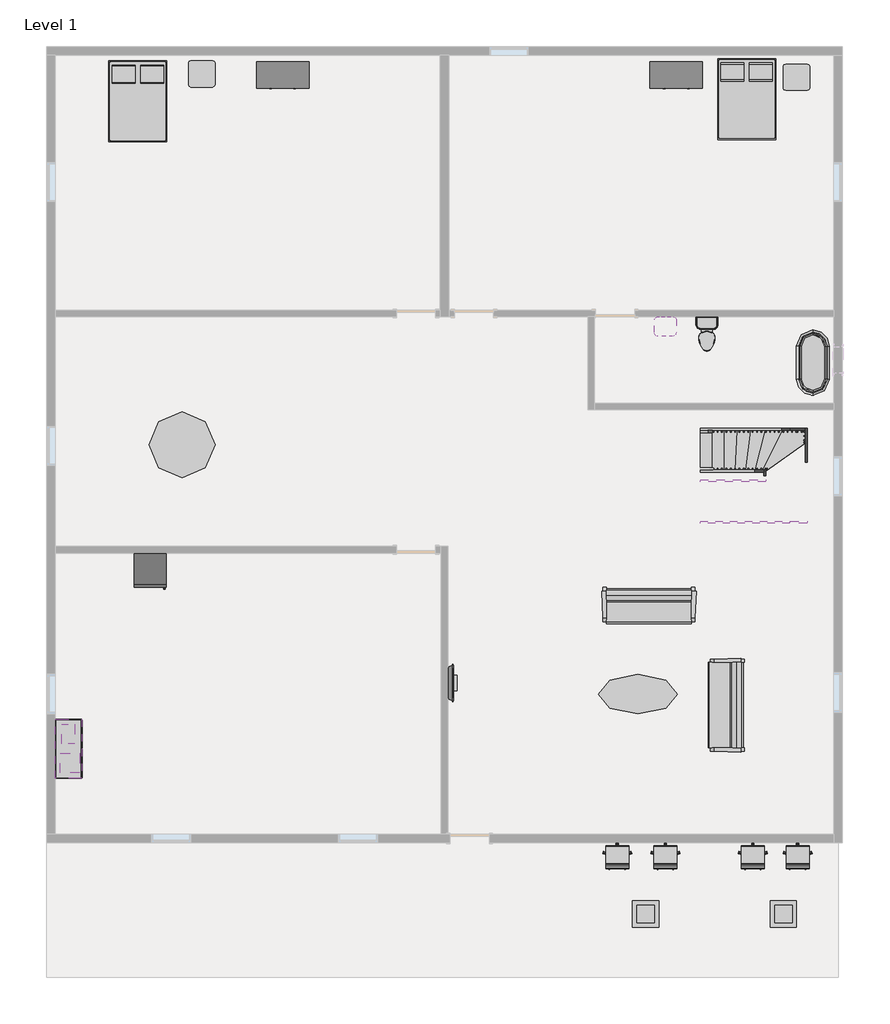
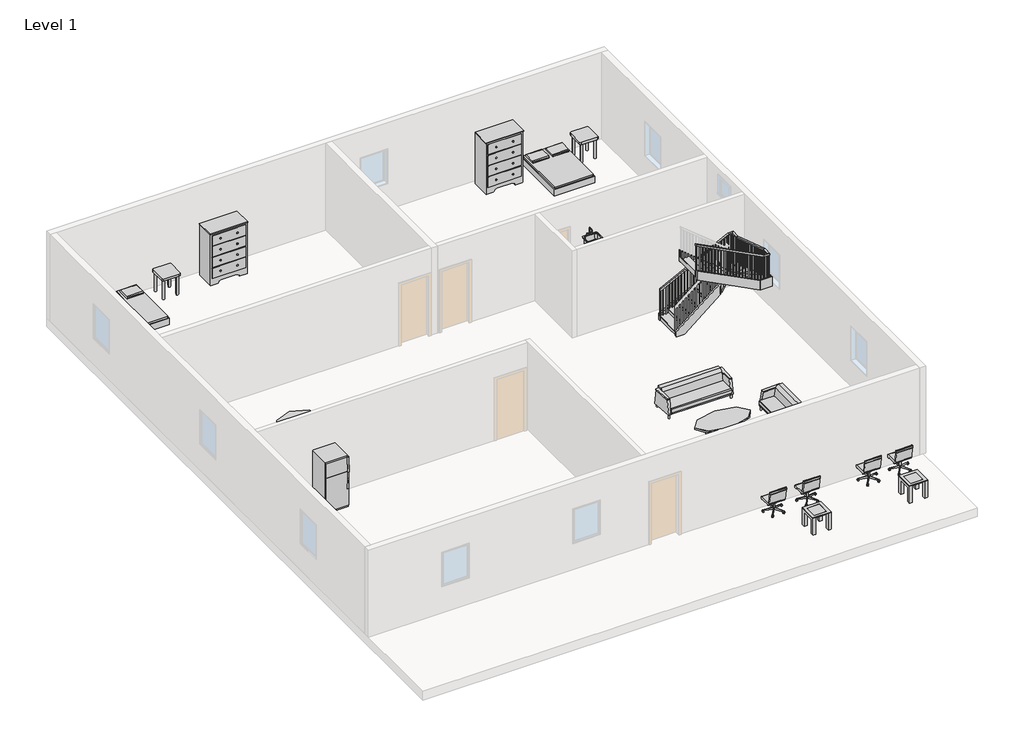
# One storey, part 2 of 2: 18 furniture elements, 8 members, 4 flow terminals, 3 proxies, 1 railing, 1 stair flight.
"""IFC4 building model written with IfcOpenShell, lengths in millimetres."""

from ifc_helpers import new_model, si_unit, frame, origin, place, context, project, spatial, polyline, outline, extrude, faceted_brep, transform, mapped, element, save
from components import proxy_fe84b772, proxy_844211aa, proxy_a13a33b2, flow_terminal_871c2e40, flow_terminal_62a433f7, toilet_domestic_3d_toilet_domestic_3d_f7549cf7, toilet_domestic_3d_toilet_domestic_3d_183bbd19, flow_terminal_b374fae2, furniture_c8abb964, chair_task_chair_task_b7f3823b, furniture_95afb093, furniture_9fa109b2, furniture_aff9b2fb, furniture_56245f3a, furniture_b5c51a22, furniture_bbcc68ce, furniture_027a2ad9, furniture_bcf351fa, stair_flight_58f01264

model = new_model("IFC4")

# Units and contexts
model_context = context("Model", 3, world=origin())
ifc_project = project(units=[si_unit("LENGTHUNIT", "METRE", prefix="MILLI")], contexts=[model_context])

# Site, building, storey
site = spatial("IfcSite", under=ifc_project)
building = spatial("IfcBuilding", under=site)
storey = spatial("IfcBuildingStorey", under=building, Name="Level 1", Elevation=0.0)

# Proxies
placement = place(None, origin())
proxy_shape = proxy_fe84b772(model_context)
element("IfcBuildingElementProxy", 1, Name="Cook Top-2 Unit : 12\" x 18\"", ObjectType="Cook Top-2 Unit : 12\" x 18\"", at=placement, inside=storey, context=model_context, shape_type="MappedRepresentation", body=[
    mapped(proxy_shape, transform((-16052.9808972, -1489.9035107, 914.4), x_axis=(-1.0000000000000002, 0.0, 0.0), y_axis=(0.0, -1.0000000000000002, 0.0), z_axis=(0.0, 0.0, 1.0))),
])
proxy_2_shape = proxy_844211aa(model_context)
element("IfcBuildingElementProxy", 2, Name="Kitchenette - Small : 54\"", ObjectType="Kitchenette - Small : 54\"", at=placement, inside=storey, context=model_context, shape_type="MappedRepresentation", body=[
    mapped(proxy_2_shape, transform((-16433.9808972, -1881.7660112, 914.4), x_axis=(0.0, 1.0000000000000002, 0.0), y_axis=(-1.0000000000000002, 0.0, 0.0), z_axis=(0.0, 0.0, 1.0))),
])
proxy_3_shape = proxy_a13a33b2(model_context)
element("IfcBuildingElementProxy", 3, Name="Refrigerator : 30\" x 32\" RH", ObjectType="Refrigerator : 30\" x 32\" RH", at=placement, inside=storey, context=model_context, shape_type="MappedRepresentation", body=[
    mapped(proxy_3_shape, transform((-14231.7298687, 2310.5091937, 0.0), x_axis=(1.0000000000000007, 0.0, 0.0), y_axis=(0.0, 1.0000000000000007, 0.0), z_axis=(0.0, 0.0, 1.0))),
])

# Flow terminals
flow_terminal_shape = flow_terminal_871c2e40(model_context)
element("IfcFlowTerminal", 4, ObjectType="Sink Kitchen-Island : 18\" x 18\"", at=placement, inside=storey, context=model_context, shape_type="MappedRepresentation", body=[
    mapped(flow_terminal_shape, transform((-16088.7354961, -2208.9175469, 914.4), x_axis=(0.0, 1.0000000000000002, 0.0), y_axis=(-1.0000000000000002, 0.0, 0.0), z_axis=(0.0, 0.0, 1.0))),
])
flow_terminal_2_shape = flow_terminal_62a433f7(model_context)
element("IfcFlowTerminal", 5, ObjectType="Sink Vanity-Square : 20\" x 18\"", at=placement, inside=storey, context=model_context, shape_type="MappedRepresentation", body=[
    mapped(flow_terminal_2_shape, transform((-2276.4701378, 7989.8262926, 914.4), x_axis=(1.0, 0.0, 0.0), y_axis=(0.0, 1.0, 0.0), z_axis=(0.0, 0.0, 1.0))),
])
toilet_domestic_3d_toilet_domestic_3d_shape = toilet_domestic_3d_toilet_domestic_3d_f7549cf7(model_context)
toilet_domestic_3d_toilet_domestic_3d_2_shape = toilet_domestic_3d_toilet_domestic_3d_183bbd19(model_context)
element("IfcFlowTerminal", 6, ObjectType="Toilet-Domestic-3D : Toilet-Domestic-3D", at=placement, inside=storey, context=model_context, shape_type="MappedRepresentation", body=[
    mapped(toilet_domestic_3d_toilet_domestic_3d_shape, transform((-1295.5808972, 7675.2756664, 0.0), x_axis=(1.0, 0.0, 0.0), y_axis=(0.0, 1.0, 0.0), z_axis=(0.0, 0.0, 1.0))),
    mapped(toilet_domestic_3d_toilet_domestic_3d_2_shape, transform((-1295.5808972, 7675.2756664, 0.0), x_axis=(1.0, 0.0, 0.0), y_axis=(0.0, 1.0, 0.0), z_axis=(0.0, 0.0, 1.0))),
])
flow_terminal_3_shape = flow_terminal_b374fae2(model_context)
element("IfcFlowTerminal", 7, ObjectType="Tub-Free Standing-3D : 30\" x 60\"", at=placement, inside=storey, context=model_context, shape_type="MappedRepresentation", body=[
    mapped(flow_terminal_3_shape, transform((1168.2191028, 7103.1716937, 0.0), x_axis=(1.0, 0.0, 0.0), y_axis=(0.0, 1.0, 0.0), z_axis=(0.0, 0.0, 1.0))),
])

# Furniture
furniture_shape = furniture_c8abb964(model_context)
element("IfcFurniture", 8, ObjectType="Bed-Box : Double 53\" x 74\"", at=placement, inside=storey, context=model_context, shape_type="MappedRepresentation", body=[
    mapped(furniture_shape, transform((-14855.4333562, 13408.2012019, 0.0), x_axis=(1.0000000000000007, 0.0, 0.0), y_axis=(0.0, 1.0000000000000007, 0.0), z_axis=(0.0, 0.0, 1.0))),
])
element("IfcFurniture", 9, ObjectType="Bed-Box : Double 53\" x 74\"", at=placement, inside=storey, context=model_context, shape_type="MappedRepresentation", body=[
    mapped(furniture_shape, transform((-707.6333562, 13459.0012019, 0.0), x_axis=(1.0, 0.0, 0.0), y_axis=(0.0, 1.0, 0.0), z_axis=(0.0, 0.0, 1.0))),
])
chair_task_chair_task_shape = chair_task_chair_task_b7f3823b(model_context)
element("IfcFurniture", 10, ObjectType="Chair-Task : Chair-Task", at=placement, inside=storey, context=model_context, shape_type="MappedRepresentation", body=[
    mapped(chair_task_chair_task_shape, transform((-2401.7717169, -4396.5742079, 0.0), x_axis=(1.0, 0.0, 0.0), y_axis=(0.0, 1.0, 0.0), z_axis=(0.0, 0.0, 1.0))),
])
element("IfcFurniture", 11, ObjectType="Chair-Task : Chair-Task", at=placement, inside=storey, context=model_context, shape_type="MappedRepresentation", body=[
    mapped(chair_task_chair_task_shape, transform((-3519.3717169, -4396.5742079, 0.0), x_axis=(1.0, 0.0, 0.0), y_axis=(0.0, 1.0, 0.0), z_axis=(0.0, 0.0, 1.0))),
])
element("IfcFurniture", 12, ObjectType="Chair-Task : Chair-Task", at=placement, inside=storey, context=model_context, shape_type="MappedRepresentation", body=[
    mapped(chair_task_chair_task_shape, transform((-369.7717169, -4396.5742079, 0.0), x_axis=(1.0, 0.0, 0.0), y_axis=(0.0, 1.0, 0.0), z_axis=(0.0, 0.0, 1.0))),
])
element("IfcFurniture", 13, ObjectType="Chair-Task : Chair-Task", at=placement, inside=storey, context=model_context, shape_type="MappedRepresentation", body=[
    mapped(chair_task_chair_task_shape, transform((671.6282831, -4396.5742079, 0.0), x_axis=(1.0, 0.0, 0.0), y_axis=(0.0, 1.0, 0.0), z_axis=(0.0, 0.0, 1.0))),
])
furniture_2_shape = furniture_95afb093(model_context)
element("IfcFurniture", 14, ObjectType="Counter Top w Sink Hole : 24\" Depth", at=placement, inside=storey, context=model_context, shape_type="MappedRepresentation", body=[
    mapped(furniture_2_shape, transform((-16433.9808972, -1348.3660112, 914.4), x_axis=(0.0, 1.0000000000000002, 0.0), y_axis=(-1.0000000000000002, 0.0, 0.0), z_axis=(0.0, 0.0, 1.0))),
])
furniture_3_shape = furniture_9fa109b2(model_context)
element("IfcFurniture", 15, ObjectType="Dresser : 48\" x 72\" x 24\"", at=placement, inside=storey, context=model_context, shape_type="MappedRepresentation", body=[
    mapped(furniture_3_shape, transform((-10881.5876374, 14146.5346478, 0.0), x_axis=(1.0, 0.0, 0.0), y_axis=(0.0, 1.0, 0.0), z_axis=(0.0, 0.0, 1.0))),
])
element("IfcFurniture", 16, ObjectType="Dresser : 48\" x 72\" x 24\"", at=placement, inside=storey, context=model_context, shape_type="MappedRepresentation", body=[
    mapped(furniture_3_shape, transform((-1737.5876374, 14146.5346478, 0.0), x_axis=(1.0, 0.0, 0.0), y_axis=(0.0, 1.0, 0.0), z_axis=(0.0, 0.0, 1.0))),
])
furniture_4_shape = furniture_aff9b2fb(model_context)
element("IfcFurniture", 17, ObjectType="Sofa-Pensi : 84\"", at=placement, inside=storey, context=model_context, shape_type="MappedRepresentation", body=[
    mapped(furniture_4_shape, transform((-2920.3871472, 1187.2618576, 0.0), x_axis=(1.0, 0.0, 0.0), y_axis=(0.0, 1.0, 0.0), z_axis=(0.0, 0.0, 1.0))),
])
element("IfcFurniture", 18, ObjectType="Sofa-Pensi : 84\"", at=placement, inside=storey, context=model_context, shape_type="MappedRepresentation", body=[
    mapped(furniture_4_shape, transform((-1115.4907333, -568.4220563, 0.0), x_axis=(0.0, -1.0000000000000004, 0.0), y_axis=(1.0000000000000004, 0.0, 0.0), z_axis=(0.0, 0.0, 1.0))),
])
furniture_5_shape = furniture_56245f3a(model_context)
element("IfcFurniture", 19, ObjectType="TV - Flat Screen : 32\"", at=placement, inside=storey, context=model_context, shape_type="MappedRepresentation", body=[
    mapped(furniture_5_shape, transform((-7256.8422736, -328.7337922, 914.4), x_axis=(0.0, 1.0000000000000002, 0.0), y_axis=(-1.0000000000000002, 0.0, 0.0), z_axis=(0.0, 0.0, 1.0))),
])
furniture_6_shape = furniture_b5c51a22(model_context)
element("IfcFurniture", 20, ObjectType="Table-Coffee : 24\" x 24\" x 24\"", at=placement, inside=storey, context=model_context, shape_type="MappedRepresentation", body=[
    mapped(furniture_6_shape, transform((464.1533361, -5793.6393841, 0.0), x_axis=(1.0, 0.0, 0.0), y_axis=(0.0, 1.0, 0.0), z_axis=(0.0, 0.0, 1.0))),
])
element("IfcFurniture", 21, ObjectType="Table-Coffee : 24\" x 24\" x 24\"", at=placement, inside=storey, context=model_context, shape_type="MappedRepresentation", body=[
    mapped(furniture_6_shape, transform((-2736.2466639, -5793.6393841, 0.0), x_axis=(1.0, 0.0, 0.0), y_axis=(0.0, 1.0, 0.0), z_axis=(0.0, 0.0, 1.0))),
])
furniture_7_shape = furniture_bbcc68ce(model_context)
element("IfcFurniture", 22, ObjectType="Table-Dining Round w Chairs : 60\" Diameter", at=placement, inside=storey, context=model_context, shape_type="MappedRepresentation", body=[
    mapped(furniture_7_shape, transform((-13591.2628644, 5383.0503822, 0.0), x_axis=(1.0, 0.0, 0.0), y_axis=(0.0, 1.0, 0.0), z_axis=(0.0, 0.0, 1.0))),
])
furniture_8_shape = furniture_027a2ad9(model_context)
element("IfcFurniture", 23, ObjectType="Table-Ellipse : 72\" x 36\"", at=placement, inside=storey, context=model_context, shape_type="MappedRepresentation", body=[
    mapped(furniture_8_shape, transform((-2895.7808972, -593.0283063, 0.0), x_axis=(1.0, 0.0, 0.0), y_axis=(0.0, 1.0, 0.0), z_axis=(0.0, 0.0, 1.0))),
])
furniture_9_shape = furniture_bcf351fa(model_context)
element("IfcFurniture", 24, ObjectType="Table-End : 24\" x 24\"", at=placement, inside=storey, context=model_context, shape_type="MappedRepresentation", body=[
    mapped(furniture_9_shape, transform((-13338.9145275, 13656.3716937, 0.0), x_axis=(1.0, 0.0, 0.0), y_axis=(0.0, 1.0, 0.0), z_axis=(0.0, 0.0, 1.0))),
])
element("IfcFurniture", 25, ObjectType="Table-End : 24\" x 24\"", at=placement, inside=storey, context=model_context, shape_type="MappedRepresentation", body=[
    mapped(furniture_9_shape, transform((478.6854725, 13580.1716937, 0.0), x_axis=(1.0, 0.0, 0.0), y_axis=(0.0, 1.0, 0.0), z_axis=(0.0, 0.0, 1.0))),
])

# Members
element("IfcMember", 26, ObjectType="Stringer - 2\" Width", at=placement, inside=storey, context=model_context, shape_type="SweptSolid", body=[
    extrude(outline(polyline([(229.639954, -1451.7125891), (0.0, -1451.7125891), (0.0, -1231.9502715), (962.500629, 635.7046026), (1305.3956453, 635.7046026), (229.639954, -1451.7125891)])), frame((0.0, 5528.3716937, 0.0), z_axis=(0.0, 1.0, 0.0), x_axis=(0.0, 0.0, 1.0)), (0.0, 0.0, 1.0), 50.8),
])
element("IfcMember", 27, ObjectType="Stringer - 2\" Width", at=placement, inside=storey, context=model_context, shape_type="SweptSolid", body=[
    extrude(outline(polyline([(635.7046026, 5528.3716937), (635.7046026, 5579.1716937), (990.4191028, 5579.1716937), (990.4191028, 5528.3716937), (635.7046026, 5528.3716937)])), frame((0.0, 0.0, 962.500629), z_axis=(0.0, 0.0, 1.0), x_axis=(1.0, 0.0, 0.0)), (0.0, 0.0, 1.0), 342.8950162),
])
element("IfcMember", 28, ObjectType="Stringer - 2\" Width", at=placement, inside=storey, context=model_context, shape_type="SweptSolid", body=[
    extrude(outline(polyline([(5579.1716937, 1289.0952212), (5579.1716937, 1000.5956453), (5409.6492107, 1000.5956453), (3420.1716937, 1638.9682298), (3420.1716937, 1969.9972697), (3457.151811, 1969.9972697), (5579.1716937, 1289.0952212)])), frame((990.4191028, 0.0, 0.0), z_axis=(1.0, 0.0, 0.0), x_axis=(0.0, 1.0, 0.0)), (0.0, 0.0, 1.0), 50.8),
])
element("IfcMember", 29, ObjectType="Stringer - 2\" Width", at=placement, inside=storey, context=model_context, shape_type="SweptSolid", body=[
    extrude(outline(polyline([(1041.2191028, 3420.1716937), (1041.2191028, 3369.3716937), (635.7046026, 3369.3716937), (635.7046026, 3420.1716937), (1041.2191028, 3420.1716937)])), frame((0.0, 0.0, 1649.8904473), z_axis=(0.0, 0.0, 1.0), x_axis=(1.0, 0.0, 0.0)), (0.0, 0.0, 1.0), 320.1068224),
])
element("IfcMember", 30, ObjectType="Stringer - 2\" Width", at=placement, inside=storey, context=model_context, shape_type="SweptSolid", body=[
    extrude(outline(polyline([(1649.8904473, 635.7046026), (1969.9972697, 635.7046026), (3045.7529609, -1451.7125891), (2725.6461385, -1451.7125891), (1649.8904473, 635.7046026)])), frame((0.0, 3369.3716937, 0.0), z_axis=(0.0, 1.0, 0.0), x_axis=(0.0, 0.0, 1.0)), (0.0, 0.0, 1.0), 50.8),
])
element("IfcMember", 31, ObjectType="Stringer - 2\" Width", at=placement, inside=storey, context=model_context, shape_type="SweptSolid", body=[
    extrude(outline(polyline([(176.1764461, -1451.7125891), (0.0, -1451.7125891), (0.0, -1185.4509445), (987.1410923, 25.2191028), (1380.418648, 25.2191028), (176.1764461, -1451.7125891)])), frame((0.0, 4563.1716937, 0.0), z_axis=(0.0, 1.0, 0.0), x_axis=(0.0, 0.0, 1.0)), (0.0, 0.0, 1.0), 50.8),
])
element("IfcMember", 32, ObjectType="Stringer - 2\" Width", at=placement, inside=storey, context=model_context, shape_type="SweptSolid", body=[
    extrude(outline(polyline([(4613.9716937, 1573.2682978), (4613.9716937, 1028.5617647), (4579.7294764, 1028.5617647), (4385.3716937, 1360.465107), (4385.3716937, 1926.1409689), (4407.3345763, 1926.1409689), (4613.9716937, 1573.2682978)])), frame((25.2191028, 0.0, 0.0), z_axis=(1.0, 0.0, 0.0), x_axis=(0.0, 1.0, 0.0)), (0.0, 0.0, 1.0), 50.8),
])
element("IfcMember", 33, ObjectType="Stringer - 2\" Width", at=placement, inside=storey, context=model_context, shape_type="SweptSolid", body=[
    extrude(outline(polyline([(1532.8634131, 76.0191028), (1926.1409689, 76.0191028), (3171.8038432, -1451.7125891), (2778.5262875, -1451.7125891), (1532.8634131, 76.0191028)])), frame((0.0, 4334.5716937, 0.0), z_axis=(0.0, 1.0, 0.0), x_axis=(0.0, 0.0, 1.0)), (0.0, 0.0, 1.0), 50.8),
])

# Railing
element("IfcRailing", 34, ObjectType="Handrail - Rectangular", at=placement, inside=storey, context=model_context, shape_type="SolidModel", body=[
    faceted_brep([(-1451.7125891, 5528.3716937, 1109.0771751), (-1451.7125891, 5528.3716937, 1051.9280057), (-1451.7125891, 5477.5716937, 1051.9280057), (-1451.7125891, 5477.5716937, 1109.0771751), (808.2692674, 5528.3716937, 2273.7644996), (820.5893187, 5528.3716937, 2222.9644996), (820.5893187, 5477.5716937, 2222.9644996), (808.2692674, 5477.5716937, 2273.7644996), (990.4191028, 5528.3716937, 2273.7644996), (990.4191028, 5528.3716937, 2222.9644996), (939.6191028, 5477.5716937, 2222.9644996), (939.6191028, 5477.5716937, 2273.7644996), (990.4191028, 5251.2177411, 2273.7644996), (990.4191028, 5243.267165, 2222.9644996), (939.6191028, 5243.267165, 2222.9644996), (939.6191028, 5251.2177411, 2273.7644996), (990.4191028, 3697.3256463, 2772.3688337), (990.4191028, 3689.3750702, 2721.5688337), (939.6191028, 3689.3750702, 2721.5688337), (939.6191028, 3697.3256463, 2772.3688337), (990.4191028, 3420.1716937, 2772.3688337), (990.4191028, 3420.1716937, 2721.5688337), (939.6191028, 3470.9716937, 2721.5688337), (939.6191028, 3470.9716937, 2772.3688337), (808.2692674, 3420.1716937, 2772.3688337), (795.9492161, 3420.1716937, 2721.5688337), (795.9492161, 3470.9716937, 2721.5688337), (808.2692674, 3470.9716937, 2772.3688337), (-1451.7125891, 3420.1716937, 3937.0561582), (-1451.7125891, 3470.9716937, 3937.0561582), (-1451.7125891, 3470.9716937, 3879.9069889), (-1451.7125891, 3420.1716937, 3879.9069889)], [[[0, 1, 2, 3]], [[1, 0, 4, 5]], [[2, 1, 5, 6]], [[3, 2, 6, 7]], [[0, 3, 7, 4]], [[5, 4, 8, 9]], [[6, 5, 9, 10]], [[7, 6, 10, 11]], [[4, 7, 11, 8]], [[9, 8, 12, 13]], [[10, 9, 13, 14]], [[11, 10, 14, 15]], [[8, 11, 15, 12]], [[13, 12, 16, 17]], [[14, 13, 17, 18]], [[15, 14, 18, 19]], [[12, 15, 19, 16]], [[17, 16, 20, 21]], [[18, 17, 21, 22]], [[19, 18, 22, 23]], [[16, 19, 23, 20]], [[21, 20, 24, 25]], [[22, 21, 25, 26]], [[23, 22, 26, 27]], [[20, 23, 27, 24]], [[28, 29, 30, 31]], [[25, 24, 28, 31]], [[26, 25, 31, 30]], [[27, 26, 30, 29]], [[24, 27, 29, 28]]]),
    extrude(outline(polyline([(3872.0443296, -1436.4557326), (2878.6666667, -1436.4557326), (2878.6666667, -1417.4057326), (3862.2268642, -1417.4057326), (3872.0443296, -1436.4557326)])), frame((0.0, 3436.0466937, 0.0), z_axis=(0.0, 1.0, 0.0), x_axis=(0.0, 0.0, 1.0)), (0.0, 0.0, 1.0), 19.05),
    extrude(outline(polyline([(3819.6845145, -1334.8557326), (2878.6666667, -1334.8557326), (2878.6666667, -1315.8057326), (3809.8670491, -1315.8057326), (3819.6845145, -1334.8557326)])), frame((0.0, 3436.0466937, 0.0), z_axis=(0.0, 1.0, 0.0), x_axis=(0.0, 0.0, 1.0)), (0.0, 0.0, 1.0), 19.05),
    extrude(outline(polyline([(3767.3246993, -1233.2557326), (2878.6666667, -1233.2557326), (2878.6666667, -1214.2057326), (3757.507234, -1214.2057326), (3767.3246993, -1233.2557326)])), frame((0.0, 3436.0466937, 0.0), z_axis=(0.0, 1.0, 0.0), x_axis=(0.0, 0.0, 1.0)), (0.0, 0.0, 1.0), 19.05),
    extrude(outline(polyline([(3714.9648842, -1131.6557326), (2709.3333333, -1131.6557326), (2709.3333333, -1112.6057326), (3705.1474189, -1112.6057326), (3714.9648842, -1131.6557326)])), frame((0.0, 3436.0466937, 0.0), z_axis=(0.0, 1.0, 0.0), x_axis=(0.0, 0.0, 1.0)), (0.0, 0.0, 1.0), 19.05),
    extrude(outline(polyline([(3662.6050691, -1030.0557326), (2709.3333333, -1030.0557326), (2709.3333333, -1011.0057326), (3652.7876038, -1011.0057326), (3662.6050691, -1030.0557326)])), frame((0.0, 3436.0466937, 0.0), z_axis=(0.0, 1.0, 0.0), x_axis=(0.0, 0.0, 1.0)), (0.0, 0.0, 1.0), 19.05),
    extrude(outline(polyline([(3610.245254, -928.4557326), (2709.3333333, -928.4557326), (2709.3333333, -909.4057326), (3600.4277887, -909.4057326), (3610.245254, -928.4557326)])), frame((0.0, 3436.0466937, 0.0), z_axis=(0.0, 1.0, 0.0), x_axis=(0.0, 0.0, 1.0)), (0.0, 0.0, 1.0), 19.05),
    extrude(outline(polyline([(3557.8854389, -826.8557326), (2540.0, -826.8557326), (2540.0, -807.8057326), (3548.0679735, -807.8057326), (3557.8854389, -826.8557326)])), frame((0.0, 3436.0466937, 0.0), z_axis=(0.0, 1.0, 0.0), x_axis=(0.0, 0.0, 1.0)), (0.0, 0.0, 1.0), 19.05),
    extrude(outline(polyline([(3505.5256238, -725.2557326), (2540.0, -725.2557326), (2540.0, -706.2057326), (3495.7081584, -706.2057326), (3505.5256238, -725.2557326)])), frame((0.0, 3436.0466937, 0.0), z_axis=(0.0, 1.0, 0.0), x_axis=(0.0, 0.0, 1.0)), (0.0, 0.0, 1.0), 19.05),
    extrude(outline(polyline([(3453.1658086, -623.6557326), (2540.0, -623.6557326), (2540.0, -604.6057326), (3443.3483433, -604.6057326), (3453.1658086, -623.6557326)])), frame((0.0, 3436.0466937, 0.0), z_axis=(0.0, 1.0, 0.0), x_axis=(0.0, 0.0, 1.0)), (0.0, 0.0, 1.0), 19.05),
    extrude(outline(polyline([(3400.8059935, -522.0557326), (2370.6666667, -522.0557326), (2370.6666667, -503.0057326), (3390.9885282, -503.0057326), (3400.8059935, -522.0557326)])), frame((0.0, 3436.0466937, 0.0), z_axis=(0.0, 1.0, 0.0), x_axis=(0.0, 0.0, 1.0)), (0.0, 0.0, 1.0), 19.05),
    extrude(outline(polyline([(3348.4461784, -420.4557326), (2370.6666667, -420.4557326), (2370.6666667, -401.4057326), (3338.6287131, -401.4057326), (3348.4461784, -420.4557326)])), frame((0.0, 3436.0466937, 0.0), z_axis=(0.0, 1.0, 0.0), x_axis=(0.0, 0.0, 1.0)), (0.0, 0.0, 1.0), 19.05),
    extrude(outline(polyline([(3296.0863633, -318.8557326), (2370.6666667, -318.8557326), (2370.6666667, -299.8057326), (3286.268898, -299.8057326), (3296.0863633, -318.8557326)])), frame((0.0, 3436.0466937, 0.0), z_axis=(0.0, 1.0, 0.0), x_axis=(0.0, 0.0, 1.0)), (0.0, 0.0, 1.0), 19.05),
    extrude(outline(polyline([(3243.7265482, -217.2557326), (2201.3333333, -217.2557326), (2201.3333333, -198.2057326), (3233.9090828, -198.2057326), (3243.7265482, -217.2557326)])), frame((0.0, 3436.0466937, 0.0), z_axis=(0.0, 1.0, 0.0), x_axis=(0.0, 0.0, 1.0)), (0.0, 0.0, 1.0), 19.05),
    extrude(outline(polyline([(3191.3667331, -115.6557326), (2201.3333333, -115.6557326), (2201.3333333, -96.6057326), (3181.5492677, -96.6057326), (3191.3667331, -115.6557326)])), frame((0.0, 3436.0466937, 0.0), z_axis=(0.0, 1.0, 0.0), x_axis=(0.0, 0.0, 1.0)), (0.0, 0.0, 1.0), 19.05),
    extrude(outline(polyline([(3139.0069179, -14.0557326), (2201.3333333, -14.0557326), (2201.3333333, 4.9942674), (3129.1894526, 4.9942674), (3139.0069179, -14.0557326)])), frame((0.0, 3436.0466937, 0.0), z_axis=(0.0, 1.0, 0.0), x_axis=(0.0, 0.0, 1.0)), (0.0, 0.0, 1.0), 19.05),
    extrude(outline(polyline([(3086.6471028, 87.5442674), (2032.0, 87.5442674), (2032.0, 106.5942674), (3076.8296375, 106.5942674), (3086.6471028, 87.5442674)])), frame((0.0, 3436.0466937, 0.0), z_axis=(0.0, 1.0, 0.0), x_axis=(0.0, 0.0, 1.0)), (0.0, 0.0, 1.0), 19.05),
    extrude(outline(polyline([(3034.2872877, 189.1442674), (2032.0, 189.1442674), (2032.0, 208.1942674), (3024.4698224, 208.1942674), (3034.2872877, 189.1442674)])), frame((0.0, 3436.0466937, 0.0), z_axis=(0.0, 1.0, 0.0), x_axis=(0.0, 0.0, 1.0)), (0.0, 0.0, 1.0), 19.05),
    extrude(outline(polyline([(2981.9274726, 290.7442674), (2032.0, 290.7442674), (2032.0, 309.7942674), (2972.1100073, 309.7942674), (2981.9274726, 290.7442674)])), frame((0.0, 3436.0466937, 0.0), z_axis=(0.0, 1.0, 0.0), x_axis=(0.0, 0.0, 1.0)), (0.0, 0.0, 1.0), 19.05),
    extrude(outline(polyline([(2929.5676575, 392.3442674), (2032.0, 392.3442674), (2032.0, 411.3942674), (2919.7501921, 411.3942674), (2929.5676575, 392.3442674)])), frame((0.0, 3436.0466937, 0.0), z_axis=(0.0, 1.0, 0.0), x_axis=(0.0, 0.0, 1.0)), (0.0, 0.0, 1.0), 19.05),
    extrude(outline(polyline([(2877.2078424, 493.9442674), (1862.6666667, 493.9442674), (1862.6666667, 512.9942674), (2867.390377, 512.9942674), (2877.2078424, 493.9442674)])), frame((0.0, 3436.0466937, 0.0), z_axis=(0.0, 1.0, 0.0), x_axis=(0.0, 0.0, 1.0)), (0.0, 0.0, 1.0), 19.05),
    extrude(outline(polyline([(2824.8480272, 595.5442674), (1862.6666667, 595.5442674), (1862.6666667, 614.5942674), (2815.0305619, 614.5942674), (2824.8480272, 595.5442674)])), frame((0.0, 3436.0466937, 0.0), z_axis=(0.0, 1.0, 0.0), x_axis=(0.0, 0.0, 1.0)), (0.0, 0.0, 1.0), 19.05),
    extrude(outline(polyline([(2772.4882121, 697.1442674), (1862.6666667, 697.1442674), (1862.6666667, 716.1942674), (2762.6707468, 716.1942674), (2772.4882121, 697.1442674)])), frame((0.0, 3436.0466937, 0.0), z_axis=(0.0, 1.0, 0.0), x_axis=(0.0, 0.0, 1.0)), (0.0, 0.0, 1.0), 19.05),
    extrude(outline(polyline([(872.9441028, 3436.0466937), (853.8941028, 3436.0466937), (853.8941028, 3455.0966937), (872.9441028, 3455.0966937), (872.9441028, 3436.0466937)])), frame((0.0, 0.0, 1862.6666667), z_axis=(0.0, 0.0, 1.0), x_axis=(1.0, 0.0, 0.0)), (0.0, 0.0, 1.0), 858.902167),
    extrude(outline(polyline([(974.5441028, 3503.6506463), (974.5441028, 3484.6006463), (955.4941028, 3484.6006463), (955.4941028, 3503.6506463), (974.5441028, 3503.6506463)])), frame((0.0, 0.0, 1862.6666667), z_axis=(0.0, 0.0, 1.0), x_axis=(1.0, 0.0, 0.0)), (0.0, 0.0, 1.0), 858.902167),
    extrude(outline(polyline([(974.5441028, 3605.2506463), (974.5441028, 3586.2006463), (955.4941028, 3586.2006463), (955.4941028, 3605.2506463), (974.5441028, 3605.2506463)])), frame((0.0, 0.0, 1862.6666667), z_axis=(0.0, 0.0, 1.0), x_axis=(1.0, 0.0, 0.0)), (0.0, 0.0, 1.0), 858.902167),
    extrude(outline(polyline([(3736.7427411, 2706.3697564), (3736.7427411, 1693.3333333), (3717.6927411, 1693.3333333), (3717.6927411, 2712.4824155), (3736.7427411, 2706.3697564)])), frame((955.4941028, 0.0, 0.0), z_axis=(1.0, 0.0, 0.0), x_axis=(0.0, 1.0, 0.0)), (0.0, 0.0, 1.0), 19.05),
    extrude(outline(polyline([(3838.3427411, 2673.7689082), (3838.3427411, 1693.3333333), (3819.2927411, 1693.3333333), (3819.2927411, 2679.8815673), (3838.3427411, 2673.7689082)])), frame((955.4941028, 0.0, 0.0), z_axis=(1.0, 0.0, 0.0), x_axis=(0.0, 1.0, 0.0)), (0.0, 0.0, 1.0), 19.05),
    extrude(outline(polyline([(3939.9427411, 2641.16806), (3939.9427411, 1693.3333333), (3920.8927411, 1693.3333333), (3920.8927411, 2647.280719), (3939.9427411, 2641.16806)])), frame((955.4941028, 0.0, 0.0), z_axis=(1.0, 0.0, 0.0), x_axis=(0.0, 1.0, 0.0)), (0.0, 0.0, 1.0), 19.05),
    extrude(outline(polyline([(4041.5427411, 2608.5672118), (4041.5427411, 1693.3333333), (4022.4927411, 1693.3333333), (4022.4927411, 2614.6798708), (4041.5427411, 2608.5672118)])), frame((955.4941028, 0.0, 0.0), z_axis=(1.0, 0.0, 0.0), x_axis=(0.0, 1.0, 0.0)), (0.0, 0.0, 1.0), 19.05),
    extrude(outline(polyline([(4143.1427411, 2575.9663635), (4143.1427411, 1693.3333333), (4124.0927411, 1693.3333333), (4124.0927411, 2582.0790226), (4143.1427411, 2575.9663635)])), frame((955.4941028, 0.0, 0.0), z_axis=(1.0, 0.0, 0.0), x_axis=(0.0, 1.0, 0.0)), (0.0, 0.0, 1.0), 19.05),
    extrude(outline(polyline([(4244.7427411, 2543.3655153), (4244.7427411, 1693.3333333), (4225.6927411, 1693.3333333), (4225.6927411, 2549.4781744), (4244.7427411, 2543.3655153)])), frame((955.4941028, 0.0, 0.0), z_axis=(1.0, 0.0, 0.0), x_axis=(0.0, 1.0, 0.0)), (0.0, 0.0, 1.0), 19.05),
    extrude(outline(polyline([(4346.3427411, 2510.7646671), (4346.3427411, 1524.0), (4327.2927411, 1524.0), (4327.2927411, 2516.8773261), (4346.3427411, 2510.7646671)])), frame((955.4941028, 0.0, 0.0), z_axis=(1.0, 0.0, 0.0), x_axis=(0.0, 1.0, 0.0)), (0.0, 0.0, 1.0), 19.05),
    extrude(outline(polyline([(4447.9427411, 2478.1638189), (4447.9427411, 1524.0), (4428.8927411, 1524.0), (4428.8927411, 2484.2764779), (4447.9427411, 2478.1638189)])), frame((955.4941028, 0.0, 0.0), z_axis=(1.0, 0.0, 0.0), x_axis=(0.0, 1.0, 0.0)), (0.0, 0.0, 1.0), 19.05),
    extrude(outline(polyline([(4549.5427411, 2445.5629706), (4549.5427411, 1524.0), (4530.4927411, 1524.0), (4530.4927411, 2451.6756297), (4549.5427411, 2445.5629706)])), frame((955.4941028, 0.0, 0.0), z_axis=(1.0, 0.0, 0.0), x_axis=(0.0, 1.0, 0.0)), (0.0, 0.0, 1.0), 19.05),
    extrude(outline(polyline([(4651.1427411, 2412.9621224), (4651.1427411, 1524.0), (4632.0927411, 1524.0), (4632.0927411, 2419.0747814), (4651.1427411, 2412.9621224)])), frame((955.4941028, 0.0, 0.0), z_axis=(1.0, 0.0, 0.0), x_axis=(0.0, 1.0, 0.0)), (0.0, 0.0, 1.0), 19.05),
    extrude(outline(polyline([(4752.7427411, 2380.3612742), (4752.7427411, 1354.6666667), (4733.6927411, 1354.6666667), (4733.6927411, 2386.4739332), (4752.7427411, 2380.3612742)])), frame((955.4941028, 0.0, 0.0), z_axis=(1.0, 0.0, 0.0), x_axis=(0.0, 1.0, 0.0)), (0.0, 0.0, 1.0), 19.05),
    extrude(outline(polyline([(4854.3427411, 2347.7604259), (4854.3427411, 1354.6666667), (4835.2927411, 1354.6666667), (4835.2927411, 2353.873085), (4854.3427411, 2347.7604259)])), frame((955.4941028, 0.0, 0.0), z_axis=(1.0, 0.0, 0.0), x_axis=(0.0, 1.0, 0.0)), (0.0, 0.0, 1.0), 19.05),
    extrude(outline(polyline([(4955.9427411, 2315.1595777), (4955.9427411, 1354.6666667), (4936.8927411, 1354.6666667), (4936.8927411, 2321.2722368), (4955.9427411, 2315.1595777)])), frame((955.4941028, 0.0, 0.0), z_axis=(1.0, 0.0, 0.0), x_axis=(0.0, 1.0, 0.0)), (0.0, 0.0, 1.0), 19.05),
    extrude(outline(polyline([(5057.5427411, 2282.5587295), (5057.5427411, 1354.6666667), (5038.4927411, 1354.6666667), (5038.4927411, 2288.6713885), (5057.5427411, 2282.5587295)])), frame((955.4941028, 0.0, 0.0), z_axis=(1.0, 0.0, 0.0), x_axis=(0.0, 1.0, 0.0)), (0.0, 0.0, 1.0), 19.05),
    extrude(outline(polyline([(5159.1427411, 2249.9578813), (5159.1427411, 1354.6666667), (5140.0927411, 1354.6666667), (5140.0927411, 2256.0705403), (5159.1427411, 2249.9578813)])), frame((955.4941028, 0.0, 0.0), z_axis=(1.0, 0.0, 0.0), x_axis=(0.0, 1.0, 0.0)), (0.0, 0.0, 1.0), 19.05),
    extrude(outline(polyline([(974.5441028, 5309.2966937), (974.5441028, 5290.2466937), (955.4941028, 5290.2466937), (955.4941028, 5309.2966937), (974.5441028, 5309.2966937)])), frame((0.0, 0.0, 1185.3333333), z_axis=(0.0, 0.0, 1.0), x_axis=(1.0, 0.0, 0.0)), (0.0, 0.0, 1.0), 1037.6311663),
    extrude(outline(polyline([(974.5441028, 5410.8966937), (974.5441028, 5391.8466937), (955.4941028, 5391.8466937), (955.4941028, 5410.8966937), (974.5441028, 5410.8966937)])), frame((0.0, 0.0, 1185.3333333), z_axis=(0.0, 0.0, 1.0), x_axis=(1.0, 0.0, 0.0)), (0.0, 0.0, 1.0), 1037.6311663),
    extrude(outline(polyline([(900.3442674, 5512.4966937), (919.3942674, 5512.4966937), (919.3942674, 5493.4466937), (900.3442674, 5493.4466937), (900.3442674, 5512.4966937)])), frame((0.0, 0.0, 1185.3333333), z_axis=(0.0, 0.0, 1.0), x_axis=(1.0, 0.0, 0.0)), (0.0, 0.0, 1.0), 1037.6311663),
    extrude(outline(polyline([(2198.9352056, 773.9624109), (1185.3333333, 773.9624109), (1185.3333333, 793.0124109), (2208.752671, 793.0124109), (2198.9352056, 773.9624109)])), frame((0.0, 5493.4466937, 0.0), z_axis=(0.0, 1.0, 0.0), x_axis=(0.0, 0.0, 1.0)), (0.0, 0.0, 1.0), 19.05),
    extrude(outline(polyline([(2146.5753905, 672.3624109), (1185.3333333, 672.3624109), (1185.3333333, 691.4124109), (2156.3928558, 691.4124109), (2146.5753905, 672.3624109)])), frame((0.0, 5493.4466937, 0.0), z_axis=(0.0, 1.0, 0.0), x_axis=(0.0, 0.0, 1.0)), (0.0, 0.0, 1.0), 19.05),
    extrude(outline(polyline([(2094.2155754, 570.7624109), (1185.3333333, 570.7624109), (1185.3333333, 589.8124109), (2104.0330407, 589.8124109), (2094.2155754, 570.7624109)])), frame((0.0, 5493.4466937, 0.0), z_axis=(0.0, 1.0, 0.0), x_axis=(0.0, 0.0, 1.0)), (0.0, 0.0, 1.0), 19.05),
    extrude(outline(polyline([(2041.8557603, 469.1624109), (1185.3333333, 469.1624109), (1185.3333333, 488.2124109), (2051.6732256, 488.2124109), (2041.8557603, 469.1624109)])), frame((0.0, 5493.4466937, 0.0), z_axis=(0.0, 1.0, 0.0), x_axis=(0.0, 0.0, 1.0)), (0.0, 0.0, 1.0), 19.05),
    extrude(outline(polyline([(1989.4959452, 367.5624109), (1016.0, 367.5624109), (1016.0, 386.6124109), (1999.3134105, 386.6124109), (1989.4959452, 367.5624109)])), frame((0.0, 5493.4466937, 0.0), z_axis=(0.0, 1.0, 0.0), x_axis=(0.0, 0.0, 1.0)), (0.0, 0.0, 1.0), 19.05),
    extrude(outline(polyline([(1937.13613, 265.9624109), (1016.0, 265.9624109), (1016.0, 285.0124109), (1946.9535954, 285.0124109), (1937.13613, 265.9624109)])), frame((0.0, 5493.4466937, 0.0), z_axis=(0.0, 1.0, 0.0), x_axis=(0.0, 0.0, 1.0)), (0.0, 0.0, 1.0), 19.05),
    extrude(outline(polyline([(1884.7763149, 164.3624109), (1016.0, 164.3624109), (1016.0, 183.4124109), (1894.5937803, 183.4124109), (1884.7763149, 164.3624109)])), frame((0.0, 5493.4466937, 0.0), z_axis=(0.0, 1.0, 0.0), x_axis=(0.0, 0.0, 1.0)), (0.0, 0.0, 1.0), 19.05),
    extrude(outline(polyline([(1832.4164998, 62.7624109), (1016.0, 62.7624109), (1016.0, 81.8124109), (1842.2339651, 81.8124109), (1832.4164998, 62.7624109)])), frame((0.0, 5493.4466937, 0.0), z_axis=(0.0, 1.0, 0.0), x_axis=(0.0, 0.0, 1.0)), (0.0, 0.0, 1.0), 19.05),
    extrude(outline(polyline([(1780.0566847, -38.8375891), (846.6666667, -38.8375891), (846.6666667, -19.7875891), (1789.87415, -19.7875891), (1780.0566847, -38.8375891)])), frame((0.0, 5493.4466937, 0.0), z_axis=(0.0, 1.0, 0.0), x_axis=(0.0, 0.0, 1.0)), (0.0, 0.0, 1.0), 19.05),
    extrude(outline(polyline([(1727.6968696, -140.4375891), (846.6666667, -140.4375891), (846.6666667, -121.3875891), (1737.5143349, -121.3875891), (1727.6968696, -140.4375891)])), frame((0.0, 5493.4466937, 0.0), z_axis=(0.0, 1.0, 0.0), x_axis=(0.0, 0.0, 1.0)), (0.0, 0.0, 1.0), 19.05),
    extrude(outline(polyline([(1675.3370545, -242.0375891), (846.6666667, -242.0375891), (846.6666667, -222.9875891), (1685.1545198, -222.9875891), (1675.3370545, -242.0375891)])), frame((0.0, 5493.4466937, 0.0), z_axis=(0.0, 1.0, 0.0), x_axis=(0.0, 0.0, 1.0)), (0.0, 0.0, 1.0), 19.05),
    extrude(outline(polyline([(1622.9772393, -343.6375891), (677.3333333, -343.6375891), (677.3333333, -324.5875891), (1632.7947047, -324.5875891), (1622.9772393, -343.6375891)])), frame((0.0, 5493.4466937, 0.0), z_axis=(0.0, 1.0, 0.0), x_axis=(0.0, 0.0, 1.0)), (0.0, 0.0, 1.0), 19.05),
    extrude(outline(polyline([(1570.6174242, -445.2375891), (677.3333333, -445.2375891), (677.3333333, -426.1875891), (1580.4348896, -426.1875891), (1570.6174242, -445.2375891)])), frame((0.0, 5493.4466937, 0.0), z_axis=(0.0, 1.0, 0.0), x_axis=(0.0, 0.0, 1.0)), (0.0, 0.0, 1.0), 19.05),
    extrude(outline(polyline([(1518.2576091, -546.8375891), (677.3333333, -546.8375891), (677.3333333, -527.7875891), (1528.0750744, -527.7875891), (1518.2576091, -546.8375891)])), frame((0.0, 5493.4466937, 0.0), z_axis=(0.0, 1.0, 0.0), x_axis=(0.0, 0.0, 1.0)), (0.0, 0.0, 1.0), 19.05),
    extrude(outline(polyline([(1465.897794, -648.4375891), (508.0, -648.4375891), (508.0, -629.3875891), (1475.7152593, -629.3875891), (1465.897794, -648.4375891)])), frame((0.0, 5493.4466937, 0.0), z_axis=(0.0, 1.0, 0.0), x_axis=(0.0, 0.0, 1.0)), (0.0, 0.0, 1.0), 19.05),
    extrude(outline(polyline([(1413.5379789, -750.0375891), (508.0, -750.0375891), (508.0, -730.9875891), (1423.3554442, -730.9875891), (1413.5379789, -750.0375891)])), frame((0.0, 5493.4466937, 0.0), z_axis=(0.0, 1.0, 0.0), x_axis=(0.0, 0.0, 1.0)), (0.0, 0.0, 1.0), 19.05),
    extrude(outline(polyline([(1361.1781638, -851.6375891), (508.0, -851.6375891), (508.0, -832.5875891), (1370.9956291, -832.5875891), (1361.1781638, -851.6375891)])), frame((0.0, 5493.4466937, 0.0), z_axis=(0.0, 1.0, 0.0), x_axis=(0.0, 0.0, 1.0)), (0.0, 0.0, 1.0), 19.05),
    extrude(outline(polyline([(1308.8183486, -953.2375891), (338.6666667, -953.2375891), (338.6666667, -934.1875891), (1318.635814, -934.1875891), (1308.8183486, -953.2375891)])), frame((0.0, 5493.4466937, 0.0), z_axis=(0.0, 1.0, 0.0), x_axis=(0.0, 0.0, 1.0)), (0.0, 0.0, 1.0), 19.05),
    extrude(outline(polyline([(1256.4585335, -1054.8375891), (338.6666667, -1054.8375891), (338.6666667, -1035.7875891), (1266.2759989, -1035.7875891), (1256.4585335, -1054.8375891)])), frame((0.0, 5493.4466937, 0.0), z_axis=(0.0, 1.0, 0.0), x_axis=(0.0, 0.0, 1.0)), (0.0, 0.0, 1.0), 19.05),
    extrude(outline(polyline([(1204.0987184, -1156.4375891), (338.6666667, -1156.4375891), (338.6666667, -1137.3875891), (1213.9161837, -1137.3875891), (1204.0987184, -1156.4375891)])), frame((0.0, 5493.4466937, 0.0), z_axis=(0.0, 1.0, 0.0), x_axis=(0.0, 0.0, 1.0)), (0.0, 0.0, 1.0), 19.05),
    extrude(outline(polyline([(1151.7389033, -1258.0375891), (169.3333333, -1258.0375891), (169.3333333, -1238.9875891), (1161.5563686, -1238.9875891), (1151.7389033, -1258.0375891)])), frame((0.0, 5493.4466937, 0.0), z_axis=(0.0, 1.0, 0.0), x_axis=(0.0, 0.0, 1.0)), (0.0, 0.0, 1.0), 19.05),
    extrude(outline(polyline([(1099.3790882, -1359.6375891), (169.3333333, -1359.6375891), (169.3333333, -1340.5875891), (1109.1965535, -1340.5875891), (1099.3790882, -1359.6375891)])), frame((0.0, 5493.4466937, 0.0), z_axis=(0.0, 1.0, 0.0), x_axis=(0.0, 0.0, 1.0)), (0.0, 0.0, 1.0), 19.05),
    extrude(outline(polyline([(817.7942674, 3436.0466937), (798.7442674, 3436.0466937), (798.7442674, 3455.0966937), (817.7942674, 3455.0966937), (817.7942674, 3436.0466937)])), frame((0.0, 0.0, 1862.6666667), z_axis=(0.0, 0.0, 1.0), x_axis=(1.0, 0.0, 0.0)), (0.0, 0.0, 1.0), 858.902167),
    extrude(outline(polyline([(974.5441028, 3455.0966937), (974.5441028, 3436.0466937), (955.4941028, 3436.0466937), (955.4941028, 3455.0966937), (974.5441028, 3455.0966937)])), frame((0.0, 0.0, 1862.6666667), z_axis=(0.0, 0.0, 1.0), x_axis=(1.0, 0.0, 0.0)), (0.0, 0.0, 1.0), 858.902167),
    extrude(outline(polyline([(3706.8506463, 2715.9613671), (3706.8506463, 1862.6666667), (3687.8006463, 1862.6666667), (3687.8006463, 2722.0740262), (3706.8506463, 2715.9613671)])), frame((955.4941028, 0.0, 0.0), z_axis=(1.0, 0.0, 0.0), x_axis=(0.0, 1.0, 0.0)), (0.0, 0.0, 1.0), 19.05),
    extrude(outline(polyline([(974.5441028, 5260.7427411), (974.5441028, 5241.6927411), (955.4941028, 5241.6927411), (955.4941028, 5260.7427411), (974.5441028, 5260.7427411)])), frame((0.0, 0.0, 1185.3333333), z_axis=(0.0, 0.0, 1.0), x_axis=(1.0, 0.0, 0.0)), (0.0, 0.0, 1.0), 1037.6311663),
    extrude(outline(polyline([(955.4941028, 5512.4966937), (974.5441028, 5512.4966937), (974.5441028, 5493.4466937), (955.4941028, 5493.4466937), (955.4941028, 5512.4966937)])), frame((0.0, 0.0, 1185.3333333), z_axis=(0.0, 0.0, 1.0), x_axis=(1.0, 0.0, 0.0)), (0.0, 0.0, 1.0), 1037.6311663),
    extrude(outline(polyline([(2211.7065976, 798.7442674), (1185.3333333, 798.7442674), (1185.3333333, 817.7942674), (2221.5240629, 817.7942674), (2211.7065976, 798.7442674)])), frame((0.0, 5493.4466937, 0.0), z_axis=(0.0, 1.0, 0.0), x_axis=(0.0, 0.0, 1.0)), (0.0, 0.0, 1.0), 19.05),
    extrude(outline(polyline([(3879.9069889, -1451.7125891), (2878.6666667, -1451.7125891), (2878.6666667, -1432.6625891), (3870.0895235, -1432.6625891), (3879.9069889, -1451.7125891)])), frame((0.0, 3436.0466937, 0.0), z_axis=(0.0, 1.0, 0.0), x_axis=(0.0, 0.0, 1.0)), (0.0, 0.0, 1.0), 19.05),
    extrude(outline(polyline([(1051.9280057, -1451.7125891), (169.3333333, -1451.7125891), (169.3333333, -1432.6625891), (1061.7454711, -1432.6625891), (1051.9280057, -1451.7125891)])), frame((0.0, 5493.4466937, 0.0), z_axis=(0.0, 1.0, 0.0), x_axis=(0.0, 0.0, 1.0)), (0.0, 0.0, 1.0), 19.05),
])

# Stair flight
stair_flight_shape = stair_flight_58f01264(model_context)
element("IfcStairFlight", 35, ObjectType="2\" Tread 1\" Nosing 1/4\" Riser", at=placement, inside=storey, context=model_context, shape_type="MappedRepresentation", body=[
    mapped(stair_flight_shape, transform((0.0, 0.0, 0.0), x_axis=(1.0, 0.0, 0.0), y_axis=(0.0, 1.0, 0.0), z_axis=(0.0, 0.0, 1.0))),
])

save(model, "model.ifc")

# Revit data of these elements
# Type "Cook Top-2 Unit : 12\" x 18\""
#   Assembly Code = "E1090400"
#   Counter Height = 3' - 0"
#   Depth = 1' - 6"
#   Width = 1' - 0"
#   Burner Material = Steel, Chrome Plated
#   Cooktop Material = Steel, Polished
#   Default Elevation = 0
# Type "Kitchenette - Small : 54\""
#   Assembly Code = "E1090400"
#   Width = 4' - 6"
#   Height = 2' - 10 1/2"
#   Depth = 2' - 0"
#   Toe Depth = 0' - 3"
#   Toe Height = 0' - 3 1/2"
#   Cabinet Material = Cabinets
#   Door/Drawer Material = Cabinets
#   Handle Material = Cabinets - Handles
#   Default Elevation = 0
# Type "Refrigerator : 30\" x 32\" RH"
#   Label = "REF."
#   Assembly Code = "E1090400"
#   Depth = 2' - 7 3/4"
#   Handle = 2' - 3"
#   Height = 5' - 10"
#   Rear Clearance = 0' - 2"
#   Top Door Height = 1' - 8"
#   Width = 2' - 5 3/8"
#   Material = Steel, Paint Finish, Ivory, Glossy
#   Default Elevation = 0
# Type "Sink Kitchen-Island : 18\" x 18\""
#   Assembly Code = "D2010410"
#   Counter Height = 3' - 0"
#   Depth = 1' - 6"
#   Width = 1' - 6"
#   Faucet Material = Steel, Polished
#   Sink Material = Steel, Polished
#   Default Elevation = 0
# Type "Sink Vanity-Square : 20\" x 18\""
#   Assembly Code = "D2010400"
#   Counter Height = 2' - 7"
#   Depth = 1' - 6"
#   Width = 1' - 8"
#   Basin Material = Porcelain, Linen
#   Faucet Material = Steel, Polished
#   Default Elevation = 0
# Type "Toilet-Domestic-3D : Toilet-Domestic-3D"
#   Assembly Code = "D2010110"
#   Toilet - Bowl/Basin Material = Porcelain, Linen
#   Toilet - Seat Material = Laminate, Linen, Matte
#   Default Elevation = 0
# Type "Tub-Free Standing-3D : 30\" x 60\""
#   Assembly Code = "D2010110"
#   Height = 1' - 6"
#   Length = 5' - 0"
#   Width = 2' - 6"
#   Tub Material = Porcelain, Ivory
#   Default Elevation = 0
# Type "Bed-Box : Double 53\" x 74\""
#   Assembly Code = "E2020200"
#   Length = 6' - 2"
#   Width = 4' - 5"
#   Frame Material = Birch
#   Mattress Material = Linen, White
#   Default Elevation = 0
# Type "Chair-Task : Chair-Task"
#   Assembly Code = "E2020200"
#   Base Material = Plastic, Opaque Black
#   Caster Material = Plastic, Opaque Black
#   Seat/Back Material = Textile - Slate Blue
#   Default Elevation = 0
# Type "Counter Top w Sink Hole : 24\" Depth"
#   Assembly Code = "C1030400"
#   Counter Thickness = 0' - 1 1/2"
#   Depth [instance default] = 2' - 1"
#   Height = 3' - 0"
#   Length [instance default] = 8' - 0"
#   Sink Location [instance default] = 2' - 0"
#   Sink Location To Wall [instance default] = 0' - 6"
#   Sink Opening Depth [instance default] = 1' - 3"
#   Sink Opening Width [instance default] = 2' - 3"
#   Counter Top Material = none
#   Default Elevation = 0
# Type "Dresser : 48\" x 72\" x 24\""
#   Assembly Code = "E2020200"
#   Depth = 2' - 0"
#   Height = 6' - 0"
#   Width = 4' - 0"
#   Dresser Material = Laminate - Ivory, Glossy
#   Drawer Material = Laminate, Ivory, Matte
#   Knob Material = Cherry
#   Default Elevation = 0
# Type "Sofa-Pensi : 84\""
#   Assembly Code = "E2020200"
#   Length = 7' - 0"
#   Frame Material = Cherry
#   Seat Material = Linen, Beige
#   Feet Material = Steel, Chrome Plated
#   Default Elevation = 0
# Type "TV - Flat Screen : 32\""
#   SinAng = 0' - 0.0193"
#   L = 2' - 3.79372"
#   H = 1' - 3.6354"
#   Thickness = 0' - 4.33071"
#   Diagonal = 2' - 7.88976"
#   CosAng = 0' - 0.03431"
#   Stand [instance default] = yes
#   Default Elevation = 0
# Type "Table-Coffee : 24\" x 24\" x 24\""
#   Assembly Code = "E2020200"
#   Height = 2' - 0"
#   Length = 2' - 0"
#   Width = 2' - 0"
#   Top Material = none
#   Frame Material = none
#   Default Elevation = 0
# Type "Table-Dining Round w Chairs : 60\" Diameter"
#   Assembly Code = "E2020200"
#   Radius = 2' - 6"
#   Diameter = 5' - 0"
#   Height = 2' - 6"
#   Chairs = 6
#   Base Material = Pine
#   Top Material = Laminate, Linen, Matte
#   Default Elevation = 0
# Type "Table-Ellipse : 72\" x 36\""
#   Assembly Code = "E2020200"
#   Half Width = 1' - 6"
#   Half Length = 3' - 0"
#   Height = 2' - 6"
#   Length = 6' - 0"
#   Width = 3' - 0"
#   Base Material = Birch
#   Top Material = Laminate - Black
#   Default Elevation = 0
# Type "Table-End : 24\" x 24\""
#   Assembly Code = "E2020200"
#   Height = 2' - 6"
#   Length = 2' - 0"
#   Width = 2' - 0"
#   Base Material = Birch
#   Top Material = Laminate, Ivory, Matte
#   Default Elevation = 0
# Type "Handrail - Rectangular"
#   Assembly Code = "C2010400"
#   built-in parameter 1008612 = 0.0416667 (stored number, unit not read)
#   built-in parameter 1008611 = 0.0416667 (stored number, unit not read)
#   built-in parameter 1008609 = 0.333333 (stored number, unit not read)
#   built-in parameter 1008604 = 0.166667 (stored number, unit not read)
#   built-in parameter 1008603 = 0.166667 (stored number, unit not read)
#   Railing Height = 3' - 0"
#   built-in parameter 1008630 = 2
#   built-in parameter 1008610 = 2
#   built-in parameter 1008618 = Baluster - Square : 3/4"
# Element 1 (IfcBuildingElementProxy, "Cook Top-2 Unit : 12\" x 18\"")
#   Phase Created = New Construction
#   Materials on its faces: "Steel, Chrome Plated", "Steel, Polished"
# Element 2 (IfcBuildingElementProxy, "Kitchenette - Small : 54\"")
#   Phase Created = New Construction
#   Materials on its faces: "Cabinets", "Cabinets - Handles"
# Element 3 (IfcBuildingElementProxy, "Refrigerator : 30\" x 32\" RH")
#   Phase Created = New Construction
#   Materials on its faces: "Steel, Paint Finish, Ivory, Glossy", "Steel, Chrome Plated"
# Element 4 (IfcFlowTerminal, "Sink Kitchen-Island : 18\" x 18\"")
#   Mark = "5"
#   Phase Created = New Construction
#   Materials on its faces: "Steel, Polished"
# Element 5 (IfcFlowTerminal, "Sink Vanity-Square : 20\" x 18\"")
#   Mark = "1"
#   Phase Created = New Construction
#   Materials on its faces: "Porcelain, Linen", "Steel, Polished"
# Element 6 (IfcFlowTerminal, "Toilet-Domestic-3D : Toilet-Domestic-3D")
#   Mark = "2"
#   Phase Created = New Construction
#   Materials on its faces: "Porcelain, Linen", "Laminate, Linen, Matte"
# Element 7 (IfcFlowTerminal, "Tub-Free Standing-3D : 30\" x 60\"")
#   Mark = "3"
#   Phase Created = New Construction
#   Materials on its faces: "Porcelain, Ivory"
# Elements 8, 9 (IfcFurniture, "Bed-Box : Double 53\" x 74\"")
#   Phase Created = New Construction
#   Materials on its faces: "Birch", "Linen, White"
# Elements 10, 11, 12, 13 (IfcFurniture, "Chair-Task : Chair-Task")
#   Phase Created = New Construction
#   Materials on its faces: "Plastic, Opaque Black", "Textile - Slate Blue"
# Element 14 (IfcFurniture, "Counter Top w Sink Hole : 24\" Depth")
#   Sink Opening Depth = 1' - 3"
#   Sink Location To Wall = 0' - 6"
#   Length = 4' - 6"
#   Sink Location = 1' - 2"
#   Sink Opening Width = 1' - 4"
#   Depth = 2' - 0"
#   Phase Created = New Construction
#   Materials on its faces: "Counter Top"
# Elements 15, 16 (IfcFurniture, "Dresser : 48\" x 72\" x 24\"")
#   Phase Created = New Construction
#   Materials on its faces: "Laminate, Ivory, Matte", "Cherry", "Laminate - Ivory, Glossy"
# Elements 17, 18 (IfcFurniture, "Sofa-Pensi : 84\"")
#   Phase Created = New Construction
#   Materials on its faces: "Cherry", "Linen, Beige", "Steel, Chrome Plated"
# Element 19 (IfcFurniture, "TV - Flat Screen : 32\"")
#   Stand = yes
#   Phase Created = New Construction
#   Materials on its faces: "TV - Black", "TV - Glass", "TV - Screen"
# Elements 20, 21 (IfcFurniture, "Table-Coffee : 24\" x 24\" x 24\"")
#   Phase Created = New Construction
#   Materials on its faces: "Glass - Clear, Grey"
# Element 22 (IfcFurniture, "Table-Dining Round w Chairs : 60\" Diameter")
#   Phase Created = New Construction
#   Materials on its faces: "Pine", "Laminate, Linen, Matte"
# Element 23 (IfcFurniture, "Table-Ellipse : 72\" x 36\"")
#   Phase Created = New Construction
#   Materials on its faces: "Birch", "Laminate - Black"
# Elements 24, 25 (IfcFurniture, "Table-End : 24\" x 24\"")
#   Phase Created = New Construction
#   Materials on its faces: "Laminate, Ivory, Matte", "Birch"
# Elements 26, 27, 28, 29, 30, 31, 32, 33 (IfcMember, "Stringer - 2\" Width")
#   Phase Created = New Construction
# Element 34 (IfcRailing, "Handrail - Rectangular")
#   Phase Created = New Construction
# Element 35 (IfcStairFlight, "2\" Tread 1\" Nosing 1/4\" Riser")
#   Phase Created = New Construction
# Materials
#   "Steel, Chrome Plated": class "Metal", colour RGB 17 17 17, transparency 0, Description = "Chromiuim plated steel", Cost = 0
#   "Steel, Polished": class "Metal", colour RGB 57 57 57, transparency 0, Description = "Polished steel", Cost = 0
#   "Cabinets": colour RGB 249 249 249, transparency 0
#   "Cabinets - Handles": class "Metal", colour RGB 57 57 57, transparency 0
#   "Steel, Paint Finish, Ivory, Glossy": class "Metal", colour RGB 247 247 239, transparency 0, Description = "Steel, paint finish, ivory, glossy", Cost = 0
#   "Porcelain, Linen": class "Ceramic", colour RGB 249 239 230, transparency 0, Description = "Porcelain, linen", Cost = 0
#   "Laminate, Linen, Matte": class "Plastic", colour RGB 249 239 230, transparency 0, Description = "Plastic Laminate - Linen, Matte", Cost = 0
#   "Porcelain, Ivory": class "Ceramic", colour RGB 247 247 239, transparency 0, Description = "Porcelain, ivory", Cost = 0
#   "Birch": class "Wood", colour RGB 224 178 126, transparency 0, Description = "Betula Alleghaniensis", Cost = 0
#   "Linen, White": class "Textile", colour RGB 247 247 239, transparency 0, Description = "Linen, white", Cost = 0
#   "Plastic, Opaque Black": class "Plastic", colour RGB 0 0 0, transparency 0.7, Description = "Plastic, generic, opaque black", Cost = 0
#   "Textile - Slate Blue": class "Fabric", colour RGB 98 102 118, transparency 0
#   "Laminate - Ivory, Glossy": colour RGB 247 247 239, transparency 0
#   "Laminate, Ivory, Matte": class "Plastic", colour RGB 247 247 239, transparency 0, Description = "Plastic Laminate - Ivory, Matte", Cost = 0
#   "Cherry": class "Wood", colour RGB 226 177 128, transparency 0, Description = "Prunus Serotina", Cost = 0
#   "Linen, Beige": class "Textile", colour RGB 249 239 230, transparency 0, Description = "Linen, beige", Cost = 0
#   "Pine": class "Wood", colour RGB 223 192 134, transparency 0, Description = "Pinus Echinata", Cost = 0
#   "Laminate - Black": colour RGB 0 0 0, transparency 0
#   "Counter Top": class "Wood", colour RGB 226 177 128, transparency 0
#   "TV - Black": colour RGB 49 49 49, transparency 0
#   "TV - Glass": colour RGB 157 157 157, transparency 0.9
#   "TV - Screen": colour RGB 0 0 0, transparency 0
#   "Glass - Clear, Grey": class "Glass", colour RGB 252 255 255, transparency 0.64
